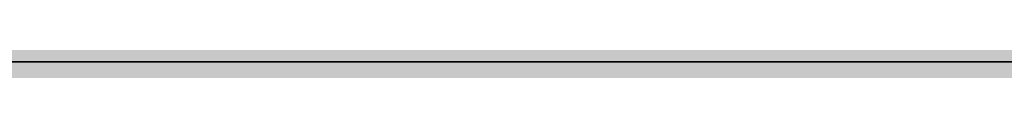
# Model space of a CAD drawing. Units: millimetres. Extents: x -22994 to 29398, y -19990 to 20176.
# Tile 91 of 135: x 229.428 to 230.597, y 83.549 to 83.564. Entities that reach past the tile are written whole.
import ezdxf
from ezdxf import colors
from ezdxf.entities.mleader import LeaderData, LeaderLine
from ezdxf.math import Vec2, Vec3

# ---------------------------------------------------------------- set-up
doc = ezdxf.new("R2010")
doc.units = ezdxf.units.MM
doc.header["$MEASUREMENT"] = 0
for name, color, linetype, lineweight in [('M-ANNO-TEXT', 7, 'Continuous', 25), ('M-DIMS', 2, 'Continuous', 18), ('M-EQPM-PATT', 7, 'Continuous', 18), ('M-PIPE', 7, 'Continuous', 35)]:
    doc.layers.add(name, color=color, linetype=linetype, lineweight=lineweight)
doc.styles.get("Standard").update_dxf_attribs({"font": 'arial.ttf'})
doc.dimstyles.get("Standard").update_dxf_attribs({"dimtxt": 0.18, "dimasz": 10000, "dimexe": 0.18, "dimexo": 0.0625, "dimgap": 0.09, "dimtad": 0, "dimtih": 1, "dimtoh": 1, "dimdec": 0, "dimzin": 0, "dimdsep": 46, "dimtxsty": 'Standard', "dimcen": 0.09, "dimadec": 0, "dimazin": 0, "dimtfac": 1, "dimtdec": 0, "dimtofl": 0, "dimtmove": 0, "dimatfit": 3, "dimfxl": 1, "dimtolj": 1, "dimtzin": 0, "dimlwd": 30, "dimarcsym": 0})

# ---------------------------------------------------------------- blocks, each defined once
blk = doc.blocks.new('*D2')
at = {"layer": 'Defpoints', "color": 0, "transparency": 16777216}
for p in [(6.6773, 10.2713), (290.852, 10.2713), (290.852, -5.0787)]:
    blk.add_point(p, dxfattribs=at)
at = {"layer": 'M-DIMS', "color": 0, "lineweight": -2, "transparency": 16777216}
for p, q in [((6.6773, 10.2088), (6.6773, -5.2587)), ((290.852, 10.2088), (290.852, -5.2587))]:
    blk.add_line(p, q, dxfattribs=at)
at = {"layer": 'M-DIMS', "color": 0, "lineweight": 30, "transparency": 16777216}
for p, q in [((-9993.3227, -5.0787), (-19993.3227, -5.0787)), ((10290.852, -5.0787), (20290.852, -5.0787))]:
    blk.add_line(p, q, dxfattribs=at)
at = {"layer": 'M-DIMS', "color": 0, "transparency": 16777216}
for points in [[(-9993.3227, 1661.5879), (-9993.3227, -1671.7454), (6.6773, -5.0787)], [(10290.852, 1661.5879), (10290.852, -1671.7454), (290.852, -5.0787)]]:
    blk.add_solid(points, dxfattribs=at)
at = {"layer": 'M-DIMS', "color": 0, "transparency": 16777216, "insert": (148.7647, -5.0787), "char_height": 0.18, "attachment_point": 5}
blk.add_mtext('\\A1;284.2', dxfattribs=at)
blk = doc.blocks.new('*D3')
at = {"layer": 'Defpoints', "color": 0, "transparency": 16777216}
for p in [(110.2647, 204.1654), (110.2647, 176.3662), (95.8327, 127.967)]:
    blk.add_point(p, dxfattribs=at)
at = {"layer": 'M-DIMS', "color": 0, "lineweight": -2, "transparency": 16777216}
for p, q in [((95.8327, 128.0295), (95.8327, 204.3454)), ((110.2647, 176.4287), (110.2647, 204.3454))]:
    blk.add_line(p, q, dxfattribs=at)
at = {"layer": 'M-DIMS', "color": 0, "lineweight": 30, "transparency": 16777216}
for p, q in [((-9904.1673, 204.1654), (-19904.1673, 204.1654)), ((10110.2647, 204.1654), (20110.2647, 204.1654))]:
    blk.add_line(p, q, dxfattribs=at)
at = {"layer": 'M-DIMS', "color": 0, "transparency": 16777216}
for points in [[(-9904.1673, 1870.8321), (-9904.1673, -1462.5013), (95.8327, 204.1654)], [(10110.2647, 1870.8321), (10110.2647, -1462.5013), (110.2647, 204.1654)]]:
    blk.add_solid(points, dxfattribs=at)
at = {"layer": 'M-DIMS', "color": 0, "transparency": 16777216, "insert": (103.0487, 204.1654), "char_height": 0.18, "attachment_point": 5}
blk.add_mtext('\\A1;14.432', dxfattribs=at)
blk = doc.blocks.new('*D4')
at = {"layer": 'Defpoints', "color": 0, "transparency": 16777216}
for p in [(116.2647, 204.1654), (110.2647, 176.3662), (116.2647, 176.3662)]:
    blk.add_point(p, dxfattribs=at)
at = {"layer": 'M-DIMS', "color": 0, "lineweight": -2, "transparency": 16777216}
for p, q in [((110.2647, 176.4287), (110.2647, 204.3454)), ((116.2647, 176.4287), (116.2647, 204.3454))]:
    blk.add_line(p, q, dxfattribs=at)
at = {"layer": 'M-DIMS', "color": 0, "lineweight": 30, "transparency": 16777216}
for p, q in [((-9889.7353, 204.1654), (-19889.7353, 204.1654)), ((10116.2647, 204.1654), (20116.2647, 204.1654))]:
    blk.add_line(p, q, dxfattribs=at)
at = {"layer": 'M-DIMS', "color": 0, "transparency": 16777216}
for points in [[(-9889.7353, 1870.8321), (-9889.7353, -1462.5013), (110.2647, 204.1654)], [(10116.2647, 1870.8321), (10116.2647, -1462.5013), (116.2647, 204.1654)]]:
    blk.add_solid(points, dxfattribs=at)
at = {"layer": 'M-DIMS', "color": 0, "transparency": 16777216, "insert": (113.2647, 204.1654), "char_height": 0.18, "attachment_point": 5}
blk.add_mtext('\\A1;6', dxfattribs=at)
blk = doc.blocks.new('*D5')
at = {"layer": 'Defpoints', "color": 0, "transparency": 16777216}
for p in [(181.2647, 204.1654), (116.2647, 176.3662), (181.2647, 176.3662)]:
    blk.add_point(p, dxfattribs=at)
at = {"layer": 'M-DIMS', "color": 0, "lineweight": -2, "transparency": 16777216}
for p, q in [((116.2647, 176.4287), (116.2647, 204.3454)), ((181.2647, 176.4287), (181.2647, 204.3454))]:
    blk.add_line(p, q, dxfattribs=at)
at = {"layer": 'M-DIMS', "color": 0, "lineweight": 30, "transparency": 16777216}
for p, q in [((-9883.7353, 204.1654), (-19883.7353, 204.1654)), ((10181.2647, 204.1654), (20181.2647, 204.1654))]:
    blk.add_line(p, q, dxfattribs=at)
at = {"layer": 'M-DIMS', "color": 0, "transparency": 16777216}
for points in [[(-9883.7353, 1870.8321), (-9883.7353, -1462.5013), (116.2647, 204.1654)], [(10181.2647, 1870.8321), (10181.2647, -1462.5013), (181.2647, 204.1654)]]:
    blk.add_solid(points, dxfattribs=at)
at = {"layer": 'M-DIMS', "color": 0, "transparency": 16777216, "insert": (148.7647, 204.1654), "char_height": 0.18, "attachment_point": 5}
blk.add_mtext('\\A1;65', dxfattribs=at)
blk = doc.blocks.new('*D6')
at = {"layer": 'Defpoints', "color": 0, "transparency": 16777216}
for p in [(187.2647, 204.1654), (181.2647, 176.3662), (187.2647, 176.3662)]:
    blk.add_point(p, dxfattribs=at)
at = {"layer": 'M-DIMS', "color": 0, "lineweight": -2, "transparency": 16777216}
for p, q in [((181.2647, 176.4287), (181.2647, 204.3454)), ((187.2647, 176.4287), (187.2647, 204.3454))]:
    blk.add_line(p, q, dxfattribs=at)
at = {"layer": 'M-DIMS', "color": 0, "lineweight": 30, "transparency": 16777216}
for p, q in [((-9818.7353, 204.1654), (-19818.7353, 204.1654)), ((10187.2647, 204.1654), (20187.2647, 204.1654))]:
    blk.add_line(p, q, dxfattribs=at)
at = {"layer": 'M-DIMS', "color": 0, "transparency": 16777216}
for points in [[(-9818.7353, 1870.8321), (-9818.7353, -1462.5013), (181.2647, 204.1654)], [(10187.2647, 1870.8321), (10187.2647, -1462.5013), (187.2647, 204.1654)]]:
    blk.add_solid(points, dxfattribs=at)
at = {"layer": 'M-DIMS', "color": 0, "transparency": 16777216, "insert": (184.2647, 204.1654), "char_height": 0.18, "attachment_point": 5}
blk.add_mtext('\\A1;6', dxfattribs=at)
blk = doc.blocks.new('*D7')
at = {"layer": 'Defpoints', "color": 0, "transparency": 16777216}
for p in [(201.6967, 204.1654), (187.2647, 176.3662), (201.6967, 127.967)]:
    blk.add_point(p, dxfattribs=at)
at = {"layer": 'M-DIMS', "color": 0, "lineweight": -2, "transparency": 16777216}
for p, q in [((187.2647, 176.4287), (187.2647, 204.3454)), ((201.6967, 128.0295), (201.6967, 204.3454))]:
    blk.add_line(p, q, dxfattribs=at)
at = {"layer": 'M-DIMS', "color": 0, "lineweight": 30, "transparency": 16777216}
for p, q in [((-9812.7353, 204.1654), (-19812.7353, 204.1654)), ((10201.6967, 204.1654), (20201.6967, 204.1654))]:
    blk.add_line(p, q, dxfattribs=at)
at = {"layer": 'M-DIMS', "color": 0, "transparency": 16777216}
for points in [[(-9812.7353, 1870.8321), (-9812.7353, -1462.5013), (187.2647, 204.1654)], [(10201.6967, 1870.8321), (10201.6967, -1462.5013), (201.6967, 204.1654)]]:
    blk.add_solid(points, dxfattribs=at)
at = {"layer": 'M-DIMS', "color": 0, "transparency": 16777216, "insert": (194.4807, 204.1654), "char_height": 0.18, "attachment_point": 5}
blk.add_mtext('\\A1;14.432', dxfattribs=at)
blk = doc.blocks.new('*D8')
at = {"layer": 'Defpoints', "color": 0, "transparency": 16777216}
for p in [(227.6485, 204.1654), (227.6485, 146.7296), (201.6967, 127.967)]:
    blk.add_point(p, dxfattribs=at)
at = {"layer": 'M-DIMS', "color": 0, "lineweight": -2, "transparency": 16777216}
for p, q in [((201.6967, 128.0295), (201.6967, 204.3454)), ((227.6485, 146.7921), (227.6485, 204.3454))]:
    blk.add_line(p, q, dxfattribs=at)
at = {"layer": 'M-DIMS', "color": 0, "lineweight": 30, "transparency": 16777216}
for p, q in [((-9798.3033, 204.1654), (-19798.3033, 204.1654)), ((10227.6485, 204.1654), (20227.6485, 204.1654))]:
    blk.add_line(p, q, dxfattribs=at)
at = {"layer": 'M-DIMS', "color": 0, "transparency": 16777216}
for points in [[(-9798.3033, 1870.8321), (-9798.3033, -1462.5013), (201.6967, 204.1654)], [(10227.6485, 1870.8321), (10227.6485, -1462.5013), (227.6485, 204.1654)]]:
    blk.add_solid(points, dxfattribs=at)
at = {"layer": 'M-DIMS', "color": 0, "transparency": 16777216, "insert": (214.6726, 204.1654), "char_height": 0.18, "attachment_point": 5}
blk.add_mtext('\\A1;25.95', dxfattribs=at)
blk = doc.blocks.new('*D9')
at = {"layer": 'Defpoints', "color": 0, "transparency": 16777216}
for p in [(187.2647, 176.3662), (306.202, 176.3662), (290.852, 10.2713)]:
    blk.add_point(p, dxfattribs=at)
at = {"layer": 'M-DIMS', "color": 0, "lineweight": 30, "transparency": 16777216}
for p, q in [((306.202, 10176.3662), (306.202, 20176.3662)), ((306.202, -9989.7287), (306.202, -19989.7287))]:
    blk.add_line(p, q, dxfattribs=at)
at = {"layer": 'M-DIMS', "color": 0, "lineweight": -2, "transparency": 16777216}
for p, q in [((187.3272, 176.3662), (306.382, 176.3662)), ((290.9145, 10.2713), (306.382, 10.2713))]:
    blk.add_line(p, q, dxfattribs=at)
at = {"layer": 'M-DIMS', "color": 0, "transparency": 16777216}
for points in [[(-1360.4646, 10176.3662), (1972.8687, 10176.3662), (306.202, 176.3662)], [(-1360.4646, -9989.7287), (1972.8687, -9989.7287), (306.202, 10.2713)]]:
    blk.add_solid(points, dxfattribs=at)
at = {"layer": 'M-DIMS', "color": 0, "transparency": 16777216, "insert": (306.202, 93.3187), "char_height": 0.18, "attachment_point": 5}
blk.add_mtext('\\A1;166.1', dxfattribs=at)
blk = doc.blocks.new('*D10')
at = {"layer": 'Defpoints', "color": 0, "transparency": 16777216}
for p in [(125.6498, 136.0713), (133.3459, 136.0713), (133.3459, -5.0787)]:
    blk.add_point(p, dxfattribs=at)
at = {"layer": 'M-DIMS', "color": 0, "lineweight": -2, "transparency": 16777216}
for p, q in [((125.6498, 136.0088), (125.6498, -5.2587)), ((133.3459, 136.0088), (133.3459, -5.2587))]:
    blk.add_line(p, q, dxfattribs=at)
at = {"layer": 'M-DIMS', "color": 0, "lineweight": 30, "transparency": 16777216}
for p, q in [((-9874.3502, -5.0787), (-19874.3502, -5.0787)), ((10133.3459, -5.0787), (20133.3459, -5.0787))]:
    blk.add_line(p, q, dxfattribs=at)
at = {"layer": 'M-DIMS', "color": 0, "transparency": 16777216}
for points in [[(-9874.3502, 1661.5879), (-9874.3502, -1671.7454), (125.6498, -5.0787)], [(10133.3459, 1661.5879), (10133.3459, -1671.7454), (133.3459, -5.0787)]]:
    blk.add_solid(points, dxfattribs=at)
at = {"layer": 'M-DIMS', "color": 0, "transparency": 16777216, "insert": (129.4978, -5.0787), "char_height": 0.18, "attachment_point": 5}
blk.add_mtext('\\A1;7.696', dxfattribs=at)
blk = doc.blocks.new('*D11')
at = {"layer": 'Defpoints', "color": 0, "transparency": 16777216}
for p in [(133.3459, 136.0713), (135.6498, 136.0713), (135.6498, -5.0787)]:
    blk.add_point(p, dxfattribs=at)
at = {"layer": 'M-DIMS', "color": 0, "lineweight": -2, "transparency": 16777216}
for p, q in [((133.3459, 136.0088), (133.3459, -5.2587)), ((135.6498, 136.0088), (135.6498, -5.2587))]:
    blk.add_line(p, q, dxfattribs=at)
at = {"layer": 'M-DIMS', "color": 0, "lineweight": 30, "transparency": 16777216}
for p, q in [((-9866.6541, -5.0787), (-19866.6541, -5.0787)), ((10135.6498, -5.0787), (20135.6498, -5.0787))]:
    blk.add_line(p, q, dxfattribs=at)
at = {"layer": 'M-DIMS', "color": 0, "transparency": 16777216}
for points in [[(-9866.6541, 1661.5879), (-9866.6541, -1671.7454), (133.3459, -5.0787)], [(10135.6498, 1661.5879), (10135.6498, -1671.7454), (135.6498, -5.0787)]]:
    blk.add_solid(points, dxfattribs=at)
at = {"layer": 'M-DIMS', "color": 0, "transparency": 16777216, "insert": (134.4978, -5.0787), "char_height": 0.18, "attachment_point": 5}
blk.add_mtext('\\A1;2.304', dxfattribs=at)
blk = doc.blocks.new('*D12')
at = {"layer": 'Defpoints', "color": 0, "transparency": 16777216}
for p in [(135.6498, 136.0713), (145.6498, 136.0713), (145.6498, -5.0787)]:
    blk.add_point(p, dxfattribs=at)
at = {"layer": 'M-DIMS', "color": 0, "lineweight": -2, "transparency": 16777216}
for p, q in [((135.6498, 136.0088), (135.6498, -5.2587)), ((145.6498, 136.0088), (145.6498, -5.2587))]:
    blk.add_line(p, q, dxfattribs=at)
at = {"layer": 'M-DIMS', "color": 0, "lineweight": 30, "transparency": 16777216}
for p, q in [((-9864.3502, -5.0787), (-19864.3502, -5.0787)), ((10145.6498, -5.0787), (20145.6498, -5.0787))]:
    blk.add_line(p, q, dxfattribs=at)
at = {"layer": 'M-DIMS', "color": 0, "transparency": 16777216}
for points in [[(-9864.3502, 1661.5879), (-9864.3502, -1671.7454), (135.6498, -5.0787)], [(10145.6498, 1661.5879), (10145.6498, -1671.7454), (145.6498, -5.0787)]]:
    blk.add_solid(points, dxfattribs=at)
at = {"layer": 'M-DIMS', "color": 0, "transparency": 16777216, "insert": (140.6498, -5.0787), "char_height": 0.18, "attachment_point": 5}
blk.add_mtext('\\A1;10', dxfattribs=at)
blk = doc.blocks.new('*D13')
at = {"layer": 'Defpoints', "color": 0, "transparency": 16777216}
for p in [(145.6498, 136.0713), (155.6498, 136.0713), (155.6498, -5.0787)]:
    blk.add_point(p, dxfattribs=at)
at = {"layer": 'M-DIMS', "color": 0, "lineweight": -2, "transparency": 16777216}
for p, q in [((145.6498, 136.0088), (145.6498, -5.2587)), ((155.6498, 136.0088), (155.6498, -5.2587))]:
    blk.add_line(p, q, dxfattribs=at)
at = {"layer": 'M-DIMS', "color": 0, "lineweight": 30, "transparency": 16777216}
for p, q in [((-9854.3502, -5.0787), (-19854.3502, -5.0787)), ((10155.6498, -5.0787), (20155.6498, -5.0787))]:
    blk.add_line(p, q, dxfattribs=at)
at = {"layer": 'M-DIMS', "color": 0, "transparency": 16777216}
for points in [[(-9854.3502, 1661.5879), (-9854.3502, -1671.7454), (145.6498, -5.0787)], [(10155.6498, 1661.5879), (10155.6498, -1671.7454), (155.6498, -5.0787)]]:
    blk.add_solid(points, dxfattribs=at)
at = {"layer": 'M-DIMS', "color": 0, "transparency": 16777216, "insert": (150.6498, -5.0787), "char_height": 0.18, "attachment_point": 5}
blk.add_mtext('\\A1;10', dxfattribs=at)
blk = doc.blocks.new('*D14')
at = {"layer": 'Defpoints', "color": 0, "transparency": 16777216}
for p in [(155.6498, 136.0713), (165.6498, 136.0713), (165.6498, -5.0787)]:
    blk.add_point(p, dxfattribs=at)
at = {"layer": 'M-DIMS', "color": 0, "lineweight": -2, "transparency": 16777216}
for p, q in [((155.6498, 136.0088), (155.6498, -5.2587)), ((165.6498, 136.0088), (165.6498, -5.2587))]:
    blk.add_line(p, q, dxfattribs=at)
at = {"layer": 'M-DIMS', "color": 0, "lineweight": 30, "transparency": 16777216}
for p, q in [((-9844.3502, -5.0787), (-19844.3502, -5.0787)), ((10165.6498, -5.0787), (20165.6498, -5.0787))]:
    blk.add_line(p, q, dxfattribs=at)
at = {"layer": 'M-DIMS', "color": 0, "transparency": 16777216}
for points in [[(-9844.3502, 1661.5879), (-9844.3502, -1671.7454), (155.6498, -5.0787)], [(10165.6498, 1661.5879), (10165.6498, -1671.7454), (165.6498, -5.0787)]]:
    blk.add_solid(points, dxfattribs=at)
at = {"layer": 'M-DIMS', "color": 0, "transparency": 16777216, "insert": (160.6498, -5.0787), "char_height": 0.18, "attachment_point": 5}
blk.add_mtext('\\A1;10', dxfattribs=at)
blk = doc.blocks.new('*D15')
at = {"layer": 'Defpoints', "color": 0, "transparency": 16777216}
for p in [(173.3459, 154.788), (173.3459, 136.0713), (306.202, 136.0713)]:
    blk.add_point(p, dxfattribs=at)
at = {"layer": 'M-DIMS', "color": 0, "lineweight": 30, "transparency": 16777216}
for p, q in [((306.202, 10154.788), (306.202, 20154.788)), ((306.202, -9863.9287), (306.202, -19863.9287))]:
    blk.add_line(p, q, dxfattribs=at)
at = {"layer": 'M-DIMS', "color": 0, "lineweight": -2, "transparency": 16777216}
for p, q in [((173.4084, 154.788), (306.382, 154.788)), ((173.4084, 136.0713), (306.382, 136.0713))]:
    blk.add_line(p, q, dxfattribs=at)
at = {"layer": 'M-DIMS', "color": 0, "transparency": 16777216}
for points in [[(-1360.4646, 10154.788), (1972.8687, 10154.788), (306.202, 154.788)], [(-1360.4646, -9863.9287), (1972.8687, -9863.9287), (306.202, 136.0713)]]:
    blk.add_solid(points, dxfattribs=at)
at = {"layer": 'M-DIMS', "color": 0, "transparency": 16777216, "insert": (306.202, 145.4297), "char_height": 0.18, "attachment_point": 5}
blk.add_mtext('\\A1;18.717', dxfattribs=at)
blk = doc.blocks.new('*D16')
at = {"layer": 'Defpoints', "color": 0, "transparency": 16777216}
for p in [(120.1702, 204.1654), (110.4658, 48.0349), (120.1702, 48.0349)]:
    blk.add_point(p, dxfattribs=at)
at = {"layer": 'M-DIMS', "color": 0, "lineweight": -2, "transparency": 16777216}
for p, q in [((110.4658, 48.0974), (110.4658, 204.3454)), ((120.1702, 48.0974), (120.1702, 204.3454))]:
    blk.add_line(p, q, dxfattribs=at)
at = {"layer": 'M-DIMS', "color": 0, "lineweight": 30, "transparency": 16777216}
for p, q in [((-9889.5342, 204.1654), (-19889.5342, 204.1654)), ((10120.1702, 204.1654), (20120.1702, 204.1654))]:
    blk.add_line(p, q, dxfattribs=at)
at = {"layer": 'M-DIMS', "color": 0, "transparency": 16777216}
for points in [[(-9889.5342, 1870.8321), (-9889.5342, -1462.5013), (110.4658, 204.1654)], [(10120.1702, 1870.8321), (10120.1702, -1462.5013), (120.1702, 204.1654)]]:
    blk.add_solid(points, dxfattribs=at)
at = {"layer": 'M-DIMS', "color": 0, "transparency": 16777216, "insert": (115.318, 204.1654), "char_height": 0.18, "attachment_point": 5}
blk.add_mtext('\\A1;9.704', dxfattribs=at)
blk = doc.blocks.new('*D17')
at = {"layer": 'Defpoints', "color": 0, "transparency": 16777216}
for p in [(126.1702, 204.1654), (120.1702, 48.0349), (126.1702, 48.0349)]:
    blk.add_point(p, dxfattribs=at)
at = {"layer": 'M-DIMS', "color": 0, "lineweight": -2, "transparency": 16777216}
for p, q in [((120.1702, 48.0974), (120.1702, 204.3454)), ((126.1702, 48.0974), (126.1702, 204.3454))]:
    blk.add_line(p, q, dxfattribs=at)
at = {"layer": 'M-DIMS', "color": 0, "lineweight": 30, "transparency": 16777216}
for p, q in [((-9879.8298, 204.1654), (-19879.8298, 204.1654)), ((10126.1702, 204.1654), (20126.1702, 204.1654))]:
    blk.add_line(p, q, dxfattribs=at)
at = {"layer": 'M-DIMS', "color": 0, "transparency": 16777216}
for points in [[(-9879.8298, 1870.8321), (-9879.8298, -1462.5013), (120.1702, 204.1654)], [(10126.1702, 1870.8321), (10126.1702, -1462.5013), (126.1702, 204.1654)]]:
    blk.add_solid(points, dxfattribs=at)
at = {"layer": 'M-DIMS', "color": 0, "transparency": 16777216, "insert": (123.1702, 204.1654), "char_height": 0.18, "attachment_point": 5}
blk.add_mtext('\\A1;6', dxfattribs=at)
blk = doc.blocks.new('*D18')
at = {"layer": 'Defpoints', "color": 0, "transparency": 16777216}
for p in [(132.1702, 204.1654), (126.1702, 48.0349), (132.1702, 48.0349)]:
    blk.add_point(p, dxfattribs=at)
at = {"layer": 'M-DIMS', "color": 0, "lineweight": -2, "transparency": 16777216}
for p, q in [((126.1702, 48.0974), (126.1702, 204.3454)), ((132.1702, 48.0974), (132.1702, 204.3454))]:
    blk.add_line(p, q, dxfattribs=at)
at = {"layer": 'M-DIMS', "color": 0, "lineweight": 30, "transparency": 16777216}
for p, q in [((-9873.8298, 204.1654), (-19873.8298, 204.1654)), ((10132.1702, 204.1654), (20132.1702, 204.1654))]:
    blk.add_line(p, q, dxfattribs=at)
at = {"layer": 'M-DIMS', "color": 0, "transparency": 16777216}
for points in [[(-9873.8298, 1870.8321), (-9873.8298, -1462.5013), (126.1702, 204.1654)], [(10132.1702, 1870.8321), (10132.1702, -1462.5013), (132.1702, 204.1654)]]:
    blk.add_solid(points, dxfattribs=at)
at = {"layer": 'M-DIMS', "color": 0, "transparency": 16777216, "insert": (129.1702, 204.1654), "char_height": 0.18, "attachment_point": 5}
blk.add_mtext('\\A1;6', dxfattribs=at)
blk = doc.blocks.new('*D19')
at = {"layer": 'Defpoints', "color": 0, "transparency": 16777216}
for p in [(138.1702, 204.1654), (132.1702, 48.0349), (138.1702, 48.0349)]:
    blk.add_point(p, dxfattribs=at)
at = {"layer": 'M-DIMS', "color": 0, "lineweight": -2, "transparency": 16777216}
for p, q in [((132.1702, 48.0974), (132.1702, 204.3454)), ((138.1702, 48.0974), (138.1702, 204.3454))]:
    blk.add_line(p, q, dxfattribs=at)
at = {"layer": 'M-DIMS', "color": 0, "lineweight": 30, "transparency": 16777216}
for p, q in [((-9867.8298, 204.1654), (-19867.8298, 204.1654)), ((10138.1702, 204.1654), (20138.1702, 204.1654))]:
    blk.add_line(p, q, dxfattribs=at)
at = {"layer": 'M-DIMS', "color": 0, "transparency": 16777216}
for points in [[(-9867.8298, 1870.8321), (-9867.8298, -1462.5013), (132.1702, 204.1654)], [(10138.1702, 1870.8321), (10138.1702, -1462.5013), (138.1702, 204.1654)]]:
    blk.add_solid(points, dxfattribs=at)
at = {"layer": 'M-DIMS', "color": 0, "transparency": 16777216, "insert": (135.1702, 204.1654), "char_height": 0.18, "attachment_point": 5}
blk.add_mtext('\\A1;6', dxfattribs=at)
blk = doc.blocks.new('*D20')
at = {"layer": 'Defpoints', "color": 0, "transparency": 16777216}
for p in [(144.1702, 204.1654), (138.1702, 48.0349), (144.1702, 48.0349)]:
    blk.add_point(p, dxfattribs=at)
at = {"layer": 'M-DIMS', "color": 0, "lineweight": -2, "transparency": 16777216}
for p, q in [((138.1702, 48.0974), (138.1702, 204.3454)), ((144.1702, 48.0974), (144.1702, 204.3454))]:
    blk.add_line(p, q, dxfattribs=at)
at = {"layer": 'M-DIMS', "color": 0, "lineweight": 30, "transparency": 16777216}
for p, q in [((-9861.8298, 204.1654), (-19861.8298, 204.1654)), ((10144.1702, 204.1654), (20144.1702, 204.1654))]:
    blk.add_line(p, q, dxfattribs=at)
at = {"layer": 'M-DIMS', "color": 0, "transparency": 16777216}
for points in [[(-9861.8298, 1870.8321), (-9861.8298, -1462.5013), (138.1702, 204.1654)], [(10144.1702, 1870.8321), (10144.1702, -1462.5013), (144.1702, 204.1654)]]:
    blk.add_solid(points, dxfattribs=at)
at = {"layer": 'M-DIMS', "color": 0, "transparency": 16777216, "insert": (141.1702, 204.1654), "char_height": 0.18, "attachment_point": 5}
blk.add_mtext('\\A1;6', dxfattribs=at)
blk = doc.blocks.new('*D21')
at = {"layer": 'Defpoints', "color": 0, "transparency": 16777216}
for p in [(149.1157, 204.1654), (144.1702, 48.0349), (149.1157, 48.0349)]:
    blk.add_point(p, dxfattribs=at)
at = {"layer": 'M-DIMS', "color": 0, "lineweight": -2, "transparency": 16777216}
for p, q in [((144.1702, 48.0974), (144.1702, 204.3454)), ((149.1157, 48.0974), (149.1157, 204.3454))]:
    blk.add_line(p, q, dxfattribs=at)
at = {"layer": 'M-DIMS', "color": 0, "lineweight": 30, "transparency": 16777216}
for p, q in [((-9855.8298, 204.1654), (-19855.8298, 204.1654)), ((10149.1157, 204.1654), (20149.1157, 204.1654))]:
    blk.add_line(p, q, dxfattribs=at)
at = {"layer": 'M-DIMS', "color": 0, "transparency": 16777216}
for points in [[(-9855.8298, 1870.8321), (-9855.8298, -1462.5013), (144.1702, 204.1654)], [(10149.1157, 1870.8321), (10149.1157, -1462.5013), (149.1157, 204.1654)]]:
    blk.add_solid(points, dxfattribs=at)
at = {"layer": 'M-DIMS', "color": 0, "transparency": 16777216, "insert": (146.6429, 204.1654), "char_height": 0.18, "attachment_point": 5}
blk.add_mtext('\\A1;4.945', dxfattribs=at)
blk = doc.blocks.new('*D22')
at = {"layer": 'Defpoints', "color": 0, "transparency": 16777216}
for p in [(149.1157, 30.9895), (155.1157, 30.9895), (155.1157, -5.0787)]:
    blk.add_point(p, dxfattribs=at)
at = {"layer": 'M-DIMS', "color": 0, "lineweight": -2, "transparency": 16777216}
for p, q in [((149.1157, 30.927), (149.1157, -5.2587)), ((155.1157, 30.927), (155.1157, -5.2587))]:
    blk.add_line(p, q, dxfattribs=at)
at = {"layer": 'M-DIMS', "color": 0, "lineweight": 30, "transparency": 16777216}
for p, q in [((-9850.8843, -5.0787), (-19850.8843, -5.0787)), ((10155.1157, -5.0787), (20155.1157, -5.0787))]:
    blk.add_line(p, q, dxfattribs=at)
at = {"layer": 'M-DIMS', "color": 0, "transparency": 16777216}
for points in [[(-9850.8843, 1661.5879), (-9850.8843, -1671.7454), (149.1157, -5.0787)], [(10155.1157, 1661.5879), (10155.1157, -1671.7454), (155.1157, -5.0787)]]:
    blk.add_solid(points, dxfattribs=at)
at = {"layer": 'M-DIMS', "color": 0, "transparency": 16777216, "insert": (152.1157, -5.0787), "char_height": 0.18, "attachment_point": 5}
blk.add_mtext('\\A1;6', dxfattribs=at)
blk = doc.blocks.new('*D23')
at = {"layer": 'Defpoints', "color": 0, "transparency": 16777216}
for p in [(155.1157, 30.9895), (161.1157, 30.9895), (161.1157, -5.0787)]:
    blk.add_point(p, dxfattribs=at)
at = {"layer": 'M-DIMS', "color": 0, "lineweight": -2, "transparency": 16777216}
for p, q in [((155.1157, 30.927), (155.1157, -5.2587)), ((161.1157, 30.927), (161.1157, -5.2587))]:
    blk.add_line(p, q, dxfattribs=at)
at = {"layer": 'M-DIMS', "color": 0, "lineweight": 30, "transparency": 16777216}
for p, q in [((-9844.8843, -5.0787), (-19844.8843, -5.0787)), ((10161.1157, -5.0787), (20161.1157, -5.0787))]:
    blk.add_line(p, q, dxfattribs=at)
at = {"layer": 'M-DIMS', "color": 0, "transparency": 16777216}
for points in [[(-9844.8843, 1661.5879), (-9844.8843, -1671.7454), (155.1157, -5.0787)], [(10161.1157, 1661.5879), (10161.1157, -1671.7454), (161.1157, -5.0787)]]:
    blk.add_solid(points, dxfattribs=at)
at = {"layer": 'M-DIMS', "color": 0, "transparency": 16777216, "insert": (158.1157, -5.0787), "char_height": 0.18, "attachment_point": 5}
blk.add_mtext('\\A1;6', dxfattribs=at)
blk = doc.blocks.new('*D24')
at = {"layer": 'Defpoints', "color": 0, "transparency": 16777216}
for p in [(161.1157, 30.9895), (166.4387, 30.9895), (166.4387, -5.0787)]:
    blk.add_point(p, dxfattribs=at)
at = {"layer": 'M-DIMS', "color": 0, "lineweight": -2, "transparency": 16777216}
for p, q in [((161.1157, 30.927), (161.1157, -5.2587)), ((166.4387, 30.927), (166.4387, -5.2587))]:
    blk.add_line(p, q, dxfattribs=at)
at = {"layer": 'M-DIMS', "color": 0, "lineweight": 30, "transparency": 16777216}
for p, q in [((-9838.8843, -5.0787), (-19838.8843, -5.0787)), ((10166.4387, -5.0787), (20166.4387, -5.0787))]:
    blk.add_line(p, q, dxfattribs=at)
at = {"layer": 'M-DIMS', "color": 0, "transparency": 16777216}
for points in [[(-9838.8843, 1661.5879), (-9838.8843, -1671.7454), (161.1157, -5.0787)], [(10166.4387, 1661.5879), (10166.4387, -1671.7454), (166.4387, -5.0787)]]:
    blk.add_solid(points, dxfattribs=at)
at = {"layer": 'M-DIMS', "color": 0, "transparency": 16777216, "insert": (163.7772, -5.0787), "char_height": 0.18, "attachment_point": 5}
blk.add_mtext('\\A1;5.323', dxfattribs=at)
blk = doc.blocks.new('*D25')
at = {"layer": 'Defpoints', "color": 0, "transparency": 16777216}
for p in [(166.4387, 30.9895), (172.4387, 30.9895), (172.4387, -5.0787)]:
    blk.add_point(p, dxfattribs=at)
at = {"layer": 'M-DIMS', "color": 0, "lineweight": -2, "transparency": 16777216}
for p, q in [((166.4387, 30.927), (166.4387, -5.2587)), ((172.4387, 30.927), (172.4387, -5.2587))]:
    blk.add_line(p, q, dxfattribs=at)
at = {"layer": 'M-DIMS', "color": 0, "lineweight": 30, "transparency": 16777216}
for p, q in [((-9833.5613, -5.0787), (-19833.5613, -5.0787)), ((10172.4387, -5.0787), (20172.4387, -5.0787))]:
    blk.add_line(p, q, dxfattribs=at)
at = {"layer": 'M-DIMS', "color": 0, "transparency": 16777216}
for points in [[(-9833.5613, 1661.5879), (-9833.5613, -1671.7454), (166.4387, -5.0787)], [(10172.4387, 1661.5879), (10172.4387, -1671.7454), (172.4387, -5.0787)]]:
    blk.add_solid(points, dxfattribs=at)
at = {"layer": 'M-DIMS', "color": 0, "transparency": 16777216, "insert": (169.4387, -5.0787), "char_height": 0.18, "attachment_point": 5}
blk.add_mtext('\\A1;6', dxfattribs=at)
blk = doc.blocks.new('*D26')
at = {"layer": 'Defpoints', "color": 0, "transparency": 16777216}
for p in [(172.4387, 30.9895), (178.4387, 30.9895), (178.4387, -5.0787)]:
    blk.add_point(p, dxfattribs=at)
at = {"layer": 'M-DIMS', "color": 0, "lineweight": -2, "transparency": 16777216}
for p, q in [((172.4387, 30.927), (172.4387, -5.2587)), ((178.4387, 30.927), (178.4387, -5.2587))]:
    blk.add_line(p, q, dxfattribs=at)
at = {"layer": 'M-DIMS', "color": 0, "lineweight": 30, "transparency": 16777216}
for p, q in [((-9827.5613, -5.0787), (-19827.5613, -5.0787)), ((10178.4387, -5.0787), (20178.4387, -5.0787))]:
    blk.add_line(p, q, dxfattribs=at)
at = {"layer": 'M-DIMS', "color": 0, "transparency": 16777216}
for points in [[(-9827.5613, 1661.5879), (-9827.5613, -1671.7454), (172.4387, -5.0787)], [(10178.4387, 1661.5879), (10178.4387, -1671.7454), (178.4387, -5.0787)]]:
    blk.add_solid(points, dxfattribs=at)
at = {"layer": 'M-DIMS', "color": 0, "transparency": 16777216, "insert": (175.4387, -5.0787), "char_height": 0.18, "attachment_point": 5}
blk.add_mtext('\\A1;6', dxfattribs=at)
blk = doc.blocks.new('*D27')
at = {"layer": 'Defpoints', "color": 0, "transparency": 16777216}
for p in [(178.4387, 30.9895), (188.1175, 30.9895), (188.1175, -5.0787)]:
    blk.add_point(p, dxfattribs=at)
at = {"layer": 'M-DIMS', "color": 0, "lineweight": -2, "transparency": 16777216}
for p, q in [((178.4387, 30.927), (178.4387, -5.2587)), ((188.1175, 30.927), (188.1175, -5.2587))]:
    blk.add_line(p, q, dxfattribs=at)
at = {"layer": 'M-DIMS', "color": 0, "lineweight": 30, "transparency": 16777216}
for p, q in [((-9821.5613, -5.0787), (-19821.5613, -5.0787)), ((10188.1175, -5.0787), (20188.1175, -5.0787))]:
    blk.add_line(p, q, dxfattribs=at)
at = {"layer": 'M-DIMS', "color": 0, "transparency": 16777216}
for points in [[(-9821.5613, 1661.5879), (-9821.5613, -1671.7454), (178.4387, -5.0787)], [(10188.1175, 1661.5879), (10188.1175, -1671.7454), (188.1175, -5.0787)]]:
    blk.add_solid(points, dxfattribs=at)
at = {"layer": 'M-DIMS', "color": 0, "transparency": 16777216, "insert": (183.2781, -5.0787), "char_height": 0.18, "attachment_point": 5}
blk.add_mtext('\\A1;9.679', dxfattribs=at)
blk = doc.blocks.new('*D28')
at = {"layer": 'Defpoints', "color": 0, "transparency": 16777216}
for p in [(188.1175, 48.0349), (306.202, 48.0349), (188.1175, 30.9895)]:
    blk.add_point(p, dxfattribs=at)
at = {"layer": 'M-DIMS', "color": 0, "lineweight": 30, "transparency": 16777216}
for p, q in [((306.202, 10048.0349), (306.202, 20048.0349)), ((306.202, -9969.0105), (306.202, -19969.0105))]:
    blk.add_line(p, q, dxfattribs=at)
at = {"layer": 'M-DIMS', "color": 0, "lineweight": -2, "transparency": 16777216}
for p, q in [((188.18, 48.0349), (306.382, 48.0349)), ((188.18, 30.9895), (306.382, 30.9895))]:
    blk.add_line(p, q, dxfattribs=at)
at = {"layer": 'M-DIMS', "color": 0, "transparency": 16777216}
for points in [[(-1360.4646, 10048.0349), (1972.8687, 10048.0349), (306.202, 48.0349)], [(-1360.4646, -9969.0105), (1972.8687, -9969.0105), (306.202, 30.9895)]]:
    blk.add_solid(points, dxfattribs=at)
at = {"layer": 'M-DIMS', "color": 0, "transparency": 16777216, "insert": (306.202, 39.5122), "char_height": 0.18, "attachment_point": 5}
blk.add_mtext('\\A1;17.045', dxfattribs=at)
blk = doc.blocks.new('*D29')
at = {"layer": 'Defpoints', "color": 0, "transparency": 16777216}
for p in [(36.8006, 80.045), (64.0296, 80.045)]:
    blk.add_point(p, dxfattribs=at)
at = {"layer": 'M-DIMS', "color": 0, "lineweight": -2, "transparency": 16777216}
for p, q in [((50.4151, 79.955), (50.4151, 80.135)), ((50.3251, 80.045), (50.5051, 80.045))]:
    blk.add_line(p, q, dxfattribs=at)
at = {"layer": 'M-DIMS', "color": 0, "lineweight": 30, "transparency": 16777216}
blk.add_line((20064.0296, 80.0303), (10064.0296, 80.0377), dxfattribs=at)
at = {"layer": 'M-DIMS', "color": 0, "transparency": 16777216}
blk.add_solid([(10064.0309, 1746.7043), (10064.0284, -1586.629), (64.0296, 80.045)], dxfattribs=at)
at = {"layer": 'M-DIMS', "color": 0, "transparency": 16777216, "insert": (20064.5213, 80.0303), "char_height": 0.18, "attachment_point": 5}
blk.add_mtext('\\A1;∅27.23', dxfattribs=at)
blk = doc.blocks.new('*D30')
at = {"layer": 'Defpoints', "color": 0, "transparency": 16777216}
for p in [(216.3148, 146.7291), (238.9821, 146.73)]:
    blk.add_point(p, dxfattribs=at)
at = {"layer": 'M-DIMS', "color": 0, "lineweight": 30, "transparency": 16777216}
blk.add_line((20238.9821, 147.4959), (10238.9821, 147.1129), dxfattribs=at)
at = {"layer": 'M-DIMS', "color": 0, "lineweight": -2, "transparency": 16777216}
for p, q in [((227.6485, 146.6396), (227.6485, 146.8196)), ((227.5585, 146.7296), (227.7385, 146.7296))]:
    blk.add_line(p, q, dxfattribs=at)
at = {"layer": 'M-DIMS', "color": 0, "transparency": 16777216}
blk.add_solid([(10238.9183, 1813.7796), (10239.0459, -1519.5537), (238.9821, 146.73)], dxfattribs=at)
at = {"layer": 'M-DIMS', "color": 0, "transparency": 16777216, "insert": (20239.5436, 147.4959), "char_height": 0.18, "attachment_point": 5}
blk.add_mtext('\\A1;∅22.667', dxfattribs=at)
blk = doc.blocks.new('*D31')
at = {"layer": 'Defpoints', "color": 0, "transparency": 16777216}
for p in [(223.1641, 146.7291), (232.1328, 146.73)]:
    blk.add_point(p, dxfattribs=at)
at = {"layer": 'M-DIMS', "color": 0, "lineweight": 30, "transparency": 16777216}
blk.add_line((20232.1327, 148.6656), (10232.1328, 147.6978), dxfattribs=at)
at = {"layer": 'M-DIMS', "color": 0, "lineweight": -2, "transparency": 16777216}
for p, q in [((227.6485, 146.6396), (227.6485, 146.8196)), ((227.5585, 146.7296), (227.7385, 146.7296))]:
    blk.add_line(p, q, dxfattribs=at)
at = {"layer": 'M-DIMS', "color": 0, "transparency": 16777216}
blk.add_solid([(10231.9715, 1814.3645), (10232.2941, -1518.9688), (232.1328, 146.73)], dxfattribs=at)
at = {"layer": 'M-DIMS', "color": 0, "transparency": 16777216, "insert": (20232.6245, 148.6656), "char_height": 0.18, "attachment_point": 5}
blk.add_mtext('\\A1;∅8.969', dxfattribs=at)
blk = doc.blocks.new('*D33')
at = {"layer": 'Defpoints', "color": 0, "transparency": 16777216}
for p in [(229.5613, 154.3773), (232.9972, 153.3509)]:
    blk.add_point(p, dxfattribs=at)
at = {"layer": 'M-DIMS', "color": 0, "lineweight": -2, "transparency": 16777216}
for p, q in [((229.5613, 154.2873), (229.5613, 154.4673)), ((229.4713, 154.3773), (229.6513, 154.3773))]:
    blk.add_line(p, q, dxfattribs=at)
at = {"layer": 'M-DIMS', "color": 0, "lineweight": 30, "transparency": 16777216}
for p, q in [((19396.3388, -5570.8378), (9814.668, -2708.7434)), ((29396.3388, -5570.8378), (19396.3388, -5570.8378))]:
    blk.add_line(p, q, dxfattribs=at)
at = {"layer": 'M-DIMS', "color": 0, "transparency": 16777216}
blk.add_solid([(10291.6837, -1111.7983), (9337.6523, -4305.6886), (232.9972, 153.3509)], dxfattribs=at)
at = {"layer": 'M-DIMS', "color": 0, "transparency": 16777216, "insert": (29397.0125, -5570.8378), "char_height": 0.18, "attachment_point": 5}
blk.add_mtext('\\A1;6X R3.586', dxfattribs=at)
blk = doc.blocks.new('*D36')
at = {"layer": 'Defpoints', "color": 0, "transparency": 16777216}
for p in [(46.39, 31.3035), (46.3875, 26.5934)]:
    blk.add_point(p, dxfattribs=at)
at = {"layer": 'M-DIMS', "color": 0, "lineweight": 30, "transparency": 16777216}
for p, q in [((57.1499, 20031.3006), (51.77, 10031.302)), ((10057.1499, 20031.3006), (57.1499, 20031.3006))]:
    blk.add_line(p, q, dxfattribs=at)
at = {"layer": 'M-DIMS', "color": 0, "lineweight": -2, "transparency": 16777216}
for p, q in [((46.3887, 28.8585), (46.3887, 29.0385)), ((46.2987, 28.9485), (46.4787, 28.9485))]:
    blk.add_line(p, q, dxfattribs=at)
at = {"layer": 'M-DIMS', "color": 0, "transparency": 16777216}
blk.add_solid([(-1614.8965, 10032.1987), (1718.4364, 10030.4054), (46.39, 31.3035)], dxfattribs=at)
at = {"layer": 'M-DIMS', "color": 0, "transparency": 16777216, "insert": (10057.5542, 20031.3006), "char_height": 0.18, "attachment_point": 5}
blk.add_mtext('\\A1;∅4.71', dxfattribs=at)

msp = doc.modelspace()

# ---------------------------------------------------------------- hatches: boundary and pattern name
at = {"layer": 'M-EQPM-PATT'}
h = msp.add_hatch(color=256, dxfattribs=at)
h.set_gradient(color1=(205, 32, 39), color2=(205, 32, 39), tint=1)
h.paths.add_polyline_path([(116.2647, 150.3662), (116.2647, 170.3662), (116.2647, 176.3662), (110.2647, 176.3662), (110.2647, 152.0276), (95.8327, 127.967), (95.8327, 16.6063), (201.6967, 16.6063), (201.6967, 127.967), (187.2647, 152.0276), (187.2647, 176.3662), (181.2647, 176.3662), (181.2647, 170.3662), (181.2647, 150.3662), (195.6967, 126.3055), (195.6967, 22.6063), (101.8327, 22.6063), (101.8327, 126.3055)])
h.paths.add_polyline_path([(185.2208, 88.6347), (101.8327, 88.6347), (101.8327, 87.6347), (182.8066, 87.6347), (178.7313, 83.5594), (195.6967, 83.5594), (195.6967, 84.5594), (181.1455, 84.5594)], flags=17)
h.paths.add_polyline_path([(95.8327, 88.6347), (60.9779, 88.6347, -0.022855), (61.7178, 87.6347), (95.8327, 87.6347)])
h.paths.add_polyline_path([(215.6212, 86.5189), (215.6212, 80.5999), (220.5095, 83.5594)])
h.paths.add_polyline_path([(215.6212, 84.5594), (201.6967, 84.5594), (201.6967, 83.5594), (215.6212, 83.5594)])
h.paths.add_polyline_path([(225.3978, 86.5189), (220.5095, 83.5594), (225.3978, 80.5999)])
h.paths.add_polyline_path([(231.6256, 84.5594), (225.3978, 84.5594), (225.3978, 83.5594), (231.6256, 83.5594)])

# ---------------------------------------------------------------- linework, layer by layer
at = {"layer": 'M-PIPE'}
msp.add_line((225.3978, 83.5594), (231.6256, 83.5594), dxfattribs=at)

# ---------------------------------------------------------------- dimensions: what is measured, and where the dimension line sits
at = {"layer": 'M-DIMS'}
for base, p1, p2, override, picture, middle in [((306.202, 176.3662), (290.852, 10.2713), (187.2647, 176.3662), {"dimdec": 1, "dimlfac": 1, "dimrnd": 0, "dimzin": 0, "dimdsep": 46, "dimlunit": 2}, '*D9', (306.202, 93.3187)), ((306.202, 136.0713), (173.3459, 154.788), (173.3459, 136.0713), {"dimdec": 3, "dimlfac": 1, "dimrnd": 0, "dimzin": 0, "dimdsep": 46, "dimlunit": 2}, '*D15', (306.202, 145.4297)), ((306.202, 48.0349), (188.1175, 30.9895), (188.1175, 48.0349), {"dimdec": 3, "dimlfac": 1, "dimrnd": 0, "dimzin": 0, "dimdsep": 46, "dimlunit": 2}, '*D28', (306.202, 39.5122))]:
    dim = msp.add_linear_dim(base=base, p1=p1, p2=p2, angle=90, dimstyle='Standard', override=override, dxfattribs=at)
    dim.commit()
    dim.dimension.update_dxf_attribs({"geometry": picture, "text_midpoint": middle})
for p1, p2, override, picture, middle in [((46.3875, 26.5934), (46.39, 31.3035), {"dimdec": 2, "dimlfac": 1, "dimrnd": 0, "dimzin": 0, "dimdsep": 46, "dimlunit": 2}, '*D36', (10057.5542, 20031.3006)), ((223.1641, 146.7291), (232.1328, 146.73), {"dimdec": 3, "dimlfac": 1, "dimrnd": 0, "dimzin": 0, "dimdsep": 46, "dimlunit": 2}, '*D31', (20232.1327, 148.6656)), ((216.3148, 146.7291), (238.9821, 146.73), {"dimdec": 3, "dimlfac": 1, "dimrnd": 0, "dimzin": 0, "dimdsep": 46, "dimlunit": 2}, '*D30', (20238.9821, 147.4959))]:
    dim = msp.add_diameter_dim_2p(p1=p1, p2=p2, dimstyle='Standard', override=override, dxfattribs=at)
    dim.commit()
    dim.dimension.update_dxf_attribs({"geometry": picture, "text_midpoint": middle, "dimtype": 163})
for base, p1, p2, override, picture, middle in [((110.2647, 204.1654), (95.8327, 127.967), (110.2647, 176.3662), {"dimdec": 3, "dimlfac": 1, "dimrnd": 0, "dimzin": 0, "dimdsep": 46, "dimlunit": 2}, '*D3', (103.0487, 204.1654)), ((116.2647, 204.1654), (110.2647, 176.3662), (116.2647, 176.3662), {"dimdec": 0, "dimlfac": 1, "dimrnd": 0, "dimzin": 0, "dimdsep": 46, "dimlunit": 2}, '*D4', (113.2647, 204.1654)), ((120.1702, 204.1654), (110.4658, 48.0349), (120.1702, 48.0349), {"dimdec": 3, "dimlfac": 1, "dimrnd": 0, "dimzin": 0, "dimdsep": 46, "dimlunit": 2}, '*D16', (115.318, 204.1654)), ((181.2647, 204.1654), (116.2647, 176.3662), (181.2647, 176.3662), {"dimdec": 0, "dimlfac": 1, "dimrnd": 0, "dimzin": 0, "dimdsep": 46, "dimlunit": 2}, '*D5', (148.7647, 204.1654)), ((126.1702, 204.1654), (120.1702, 48.0349), (126.1702, 48.0349), {"dimdec": 0, "dimlfac": 1, "dimrnd": 0, "dimzin": 0, "dimdsep": 46, "dimlunit": 2}, '*D17', (123.1702, 204.1654)), ((132.1702, 204.1654), (126.1702, 48.0349), (132.1702, 48.0349), {"dimdec": 0, "dimlfac": 1, "dimrnd": 0, "dimzin": 0, "dimdsep": 46, "dimlunit": 2}, '*D18', (129.1702, 204.1654)), ((138.1702, 204.1654), (132.1702, 48.0349), (138.1702, 48.0349), {"dimdec": 0, "dimlfac": 1, "dimrnd": 0, "dimzin": 0, "dimdsep": 46, "dimlunit": 2}, '*D19', (135.1702, 204.1654)), ((144.1702, 204.1654), (138.1702, 48.0349), (144.1702, 48.0349), {"dimdec": 0, "dimlfac": 1, "dimrnd": 0, "dimzin": 0, "dimdsep": 46, "dimlunit": 2}, '*D20', (141.1702, 204.1654)), ((149.11567, 204.16539), (144.17023, 48.03494), (149.11567, 48.03494), {"dimdec": 3, "dimlfac": 1, "dimrnd": 0, "dimzin": 0, "dimdsep": 46, "dimlunit": 2}, '*D21', (146.64295, 204.16539)), ((187.2647, 204.1654), (181.2647, 176.3662), (187.2647, 176.3662), {"dimdec": 0, "dimlfac": 1, "dimrnd": 0, "dimzin": 0, "dimdsep": 46, "dimlunit": 2}, '*D6', (184.2647, 204.1654)), ((201.6967, 204.1654), (187.2647, 176.3662), (201.6967, 127.967), {"dimdec": 3, "dimlfac": 1, "dimrnd": 0, "dimzin": 0, "dimdsep": 46, "dimlunit": 2}, '*D7', (194.4807, 204.1654)), ((227.6485, 204.1654), (201.6967, 127.967), (227.6485, 146.7296), {"dimdec": 2, "dimlfac": 1, "dimrnd": 0, "dimzin": 0, "dimdsep": 46, "dimlunit": 2}, '*D8', (214.6726, 204.1654)), ((290.852, -5.0787), (6.6773, 10.2713), (290.852, 10.2713), {"dimdec": 1, "dimlfac": 1, "dimrnd": 0, "dimzin": 0, "dimdsep": 46, "dimlunit": 2}, '*D2', (148.7647, -5.0787)), ((133.3459, -5.0787), (125.6498, 136.0713), (133.3459, 136.0713), {"dimdec": 3, "dimlfac": 1, "dimrnd": 0, "dimzin": 0, "dimdsep": 46, "dimlunit": 2}, '*D10', (129.4978, -5.0787)), ((135.6498, -5.0787), (133.3459, 136.0713), (135.6498, 136.0713), {"dimdec": 3, "dimlfac": 1, "dimrnd": 0, "dimzin": 0, "dimdsep": 46, "dimlunit": 2}, '*D11', (134.4978, -5.0787)), ((145.6498, -5.0787), (135.6498, 136.0713), (145.6498, 136.0713), {"dimdec": 0, "dimlfac": 1, "dimrnd": 0, "dimzin": 0, "dimdsep": 46, "dimlunit": 2}, '*D12', (140.6498, -5.0787)), ((155.6498, -5.0787), (145.6498, 136.0713), (155.6498, 136.0713), {"dimdec": 0, "dimlfac": 1, "dimrnd": 0, "dimzin": 0, "dimdsep": 46, "dimlunit": 2}, '*D13', (150.6498, -5.0787)), ((155.1157, -5.0787), (149.1157, 30.9895), (155.1157, 30.9895), {"dimdec": 0, "dimlfac": 1, "dimrnd": 0, "dimzin": 0, "dimdsep": 46, "dimlunit": 2}, '*D22', (152.1157, -5.0787)), ((161.1157, -5.0787), (155.1157, 30.9895), (161.1157, 30.9895), {"dimdec": 0, "dimlfac": 1, "dimrnd": 0, "dimzin": 0, "dimdsep": 46, "dimlunit": 2}, '*D23', (158.1157, -5.0787)), ((165.6498, -5.0787), (155.6498, 136.0713), (165.6498, 136.0713), {"dimdec": 0, "dimlfac": 1, "dimrnd": 0, "dimzin": 0, "dimdsep": 46, "dimlunit": 2}, '*D14', (160.6498, -5.0787)), ((166.4387, -5.0787), (161.1157, 30.9895), (166.4387, 30.9895), {"dimdec": 3, "dimlfac": 1, "dimrnd": 0, "dimzin": 0, "dimdsep": 46, "dimlunit": 2}, '*D24', (163.7772, -5.0787)), ((172.4387, -5.0787), (166.4387, 30.9895), (172.4387, 30.9895), {"dimdec": 0, "dimlfac": 1, "dimrnd": 0, "dimzin": 0, "dimdsep": 46, "dimlunit": 2}, '*D25', (169.4387, -5.0787)), ((178.4387, -5.0787), (172.4387, 30.9895), (178.4387, 30.9895), {"dimdec": 0, "dimlfac": 1, "dimrnd": 0, "dimzin": 0, "dimdsep": 46, "dimlunit": 2}, '*D26', (175.4387, -5.0787)), ((188.1175, -5.0787), (178.4387, 30.9895), (188.1175, 30.9895), {"dimdec": 3, "dimlfac": 1, "dimrnd": 0, "dimzin": 0, "dimdsep": 46, "dimlunit": 2}, '*D27', (183.2781, -5.0787))]:
    dim = msp.add_linear_dim(base=base, p1=p1, p2=p2, dimstyle='Standard', override=override, dxfattribs=at)
    dim.commit()
    dim.dimension.update_dxf_attribs({"geometry": picture, "text_midpoint": middle})
dim = msp.add_diameter_dim_2p(p1=(36.8006, 80.045), p2=(64.0296, 80.045), dimstyle='Standard', override={"dimdec": 2, "dimlfac": 1, "dimrnd": 0, "dimzin": 0, "dimdsep": 46, "dimlunit": 2}, dxfattribs=at)
dim.commit()
dim.dimension.update_dxf_attribs({"geometry": '*D29', "text_midpoint": (20064.0296, 80.0303)})
dim = msp.add_radius_dim(center=(229.5613, 154.3773), mpoint=(232.9972, 153.3509), text='6X <>', dimstyle='Standard', override={"dimdec": 3, "dimlfac": 1, "dimrnd": 0, "dimzin": 0, "dimdsep": 46, "dimlunit": 2}, dxfattribs=at)
dim.commit()
dim.dimension.update_dxf_attribs({"geometry": '*D33', "text_midpoint": (29397.0125, -5570.8378)})

# ---------------------------------------------------------------- leaders
at = {"layer": 'M-ANNO-TEXT'}
ml = msp.add_multileader_mtext('Standard', dxfattribs=at)
ml.set_content('combustion chamber', color=256)
ml.set_leader_properties()
ml.build(insert=Vec2(0, 0))
ml.multileader.update_dxf_attribs({"dogleg_length": 0.36, "arrow_head_size": 200})
ctx = ml.context
ctx.base_point, ctx.char_height, ctx.arrow_head_size, ctx.landing_gap_size, ctx.plane_origin = Vec3(215.7321, 57.9149), 3, 200, 0.09, Vec3(189.1175, 57.9149)
notes = []
notes.append((ctx, [(0, (1, 1, 0), (215.3721, 57.9149), (1, 0), 0.36, [(0, [(189.1175, 57.9149)], 0, [])])]))
ctx.mtext.insert, ctx.mtext.flow_direction = Vec3(215.8221, 59.4394), 5
for ctx, leaders in notes:
    for number, flags, end, landing, length, lines in leaders:
        leader = LeaderData()
        leader.index, (leader.has_last_leader_line, leader.has_dogleg_vector, leader.attachment_direction) = number, flags
        leader.last_leader_point, leader.dogleg_vector, leader.dogleg_length = Vec3(end), Vec3(landing), length
        for number, points, colour, breaks in lines:
            line = LeaderLine()
            line.index, line.vertices, line.color, line.breaks = number, Vec3.list(points), colors.encode_raw_color(colour), breaks
            leader.lines.append(line)
        ctx.leaders.append(leader)

doc.saveas('drawing.dxf')
